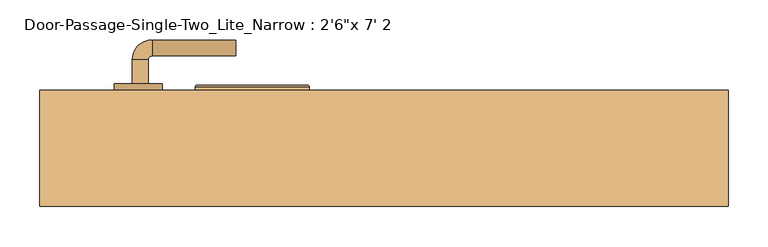
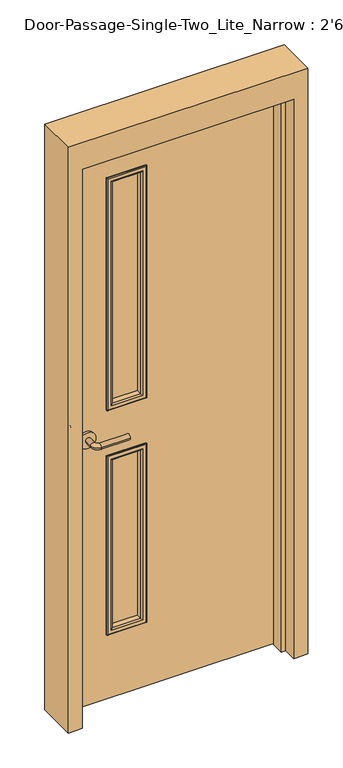
"""IFC4 building model written with IfcOpenShell, lengths in millimetres: door geometry."""

from ifc_helpers import new_model, si_unit, point, frame, frame_2d, origin, place, context, project, spatial, polyline, circle_curve, ellipse_curve, trimmed, segment, composite_curve, outline, extrude, faceted_brep, source, transform, mapped, element, save
from ifc_brep_helpers import plane_surface, cylinder_surface, revolved_surface, advanced_brep


def door_10c07981(model_context):
    return source(origin(), model_context, "Body", "SolidModel", [
        advanced_brep(
        [(-315.990625, -14.35, 1016.0), (-295.990625, -14.35, 1016.0), (-295.990625, -44.35, 1016.0), (-315.990625, -44.35, 1016.0), (-290.990625, -49.35, 1016.0), (-290.990625, -69.35, 1016.0), (-185.990625, -69.35, 1016.0), (-185.990625, -49.35, 1016.0)],
        [
            (0, 1, circle_curve(frame((-305.990625, -14.35, 1016.0), z_axis=(0.0, 1.0, 0.0), x_axis=(1.0, 0.0, 0.0)), 10.0)),
            (1, 0, circle_curve(frame((-305.990625, -14.35, 1016.0), z_axis=(0.0, 1.0, 0.0), x_axis=(1.0, 0.0, 0.0)), 10.0)),
            (1, 2),
            (2, 3, circle_curve(frame((-305.990625, -44.35, 1016.0), z_axis=(0.0, 1.0, 0.0), x_axis=(1.0, 0.0, 0.0)), 10.0)),
            (3, 0),
            (3, 2, circle_curve(frame((-305.990625, -44.35, 1016.0), z_axis=(0.0, 1.0, 0.0), x_axis=(1.0, 0.0, 0.0)), 10.0)),
            (4, 5, circle_curve(frame((-290.990625, -59.35, 1016.0), z_axis=(-1.0, 0.0, 0.0), x_axis=(0.0, 1.0, 0.0)), 10.0)),
            (5, 3, circle_curve(frame((-290.990625, -44.35, 1016.0), z_axis=(0.0, 0.0, -1.0), x_axis=(-1.0, 0.0, 0.0)), 25.0)),
            (2, 4, circle_curve(frame((-290.990625, -44.35, 1016.0), z_axis=(0.0, 0.0, 1.0), x_axis=(-1.0, 0.0, 0.0)), 5.0)),
            (5, 4, circle_curve(frame((-290.990625, -59.35, 1016.0), z_axis=(-1.0, 0.0, 0.0), x_axis=(0.0, 1.0, 0.0)), 10.0)),
            (6, 7, circle_curve(frame((-185.990625, -59.35, 1016.0), z_axis=(1.0, 0.0, 0.0), x_axis=(0.0, 1.0, 0.0)), 10.0)),
            (7, 6, circle_curve(frame((-185.990625, -59.35, 1016.0), z_axis=(1.0, 0.0, 0.0), x_axis=(0.0, 1.0, 0.0)), 10.0)),
            (4, 7),
            (6, 5),
        ],
        [
            plane_surface(frame((-305.990625, -14.35, 1016.0), z_axis=(0.0, 1.0, 0.0), x_axis=(0.0, 0.0, 1.0))),
            cylinder_surface(frame((-305.990625, -14.35, 1016.0), z_axis=(0.0, 1.0, 0.0), x_axis=(1.0, 0.0, 0.0)), 10.0),
            revolved_surface(trimmed(ellipse_curve(frame((-305.990625, -44.35, 1016.0), z_axis=(0.0, -1.0, 0.0), x_axis=(1.0, 0.0, 0.0)), 10.0, 10.0), [point((-315.990625, -44.35, 1016.0))], [point((-295.990625, -44.35, 1016.0))], True, "CARTESIAN"), (-290.990625, -44.35, 1016.0), (0.0, 0.0, -1.0)),
            revolved_surface(trimmed(ellipse_curve(frame((-305.990625, -44.35, 1016.0), z_axis=(0.0, -1.0, 0.0), x_axis=(1.0, 0.0, 0.0)), 10.0, 10.0), [point((-295.990625, -44.35, 1016.0))], [point((-315.990625, -44.35, 1016.0))], True, "CARTESIAN"), (-290.990625, -44.35, 1016.0), (0.0, 0.0, -1.0)),
            plane_surface(frame((-185.990625, -59.35, 1016.0), z_axis=(1.0, 0.0, 0.0), x_axis=(0.0, 0.0, 1.0))),
            cylinder_surface(frame((-290.990625, -59.35, 1016.0), z_axis=(-1.0, 0.0, 0.0), x_axis=(0.0, 1.0, 0.0)), 10.0),
        ],
        [
            (0, [[1, 2]]),
            (1, [[3, 4, 5, -2]]),
            (1, [[-5, 6, -3, -1]]),
            (2, [[7, 8, -4, 9]]),
            (3, [[10, -9, -6, -8]]),
            (4, [[11, 12]]),
            (5, [[13, -11, 14, -7]]),
            (5, [[-14, -12, -13, -10]]),
        ],
    ),
        extrude(outline(composite_curve([segment(trimmed(circle_curve(frame_2d((1016.0, -308.490625)), 30.0), [point((1016.0, -338.490625))], [point((1016.0, -278.490625))], False, "CARTESIAN"), True, "CONTINUOUS"), segment(trimmed(circle_curve(frame_2d((1016.0, -308.490625)), 30.0), [point((1016.0, -278.490625))], [point((1016.0, -338.490625))], False, "CARTESIAN"), True, "CONTINUOUS")], self_intersect=False)), frame((0.0, -14.35, 0.0), z_axis=(0.0, 1.0, 0.0), x_axis=(0.0, 0.0, 1.0)), (0.0, 0.0, 1.0), 8.0),
        advanced_brep(
        [(-315.990625, 46.1, 1016.0), (-295.990625, 46.1, 1016.0), (-315.990625, 76.1, 1016.0), (-295.990625, 76.1, 1016.0), (-290.990625, 81.1, 1016.0), (-290.990625, 101.1, 1016.0), (-185.990625, 101.1, 1016.0), (-185.990625, 81.1, 1016.0)],
        [
            (0, 1, circle_curve(frame((-305.990625, 46.1, 1016.0), z_axis=(0.0, -1.0, 0.0), x_axis=(1.0, 0.0, 0.0)), 10.0)),
            (1, 0, circle_curve(frame((-305.990625, 46.1, 1016.0), z_axis=(0.0, -1.0, 0.0), x_axis=(1.0, 0.0, 0.0)), 10.0)),
            (0, 2),
            (2, 3, circle_curve(frame((-305.990625, 76.1, 1016.0), z_axis=(0.0, -1.0, 0.0), x_axis=(1.0, 0.0, 0.0)), 10.0)),
            (3, 1),
            (3, 2, circle_curve(frame((-305.990625, 76.1, 1016.0), z_axis=(0.0, -1.0, 0.0), x_axis=(1.0, 0.0, 0.0)), 10.0)),
            (4, 3, circle_curve(frame((-290.990625, 76.1, 1016.0), z_axis=(0.0, 0.0, 1.0), x_axis=(-1.0, 0.0, 0.0)), 5.0)),
            (2, 5, circle_curve(frame((-290.990625, 76.1, 1016.0), z_axis=(0.0, 0.0, -1.0), x_axis=(-1.0, 0.0, 0.0)), 25.0)),
            (5, 4, circle_curve(frame((-290.990625, 91.1, 1016.0), z_axis=(-1.0, 0.0, 0.0), x_axis=(0.0, -1.0, 0.0)), 10.0)),
            (4, 5, circle_curve(frame((-290.990625, 91.1, 1016.0), z_axis=(-1.0, 0.0, 0.0), x_axis=(0.0, -1.0, 0.0)), 10.0)),
            (6, 7, circle_curve(frame((-185.990625, 91.1, 1016.0), z_axis=(1.0, 0.0, 0.0), x_axis=(0.0, -1.0, 0.0)), 10.0)),
            (7, 6, circle_curve(frame((-185.990625, 91.1, 1016.0), z_axis=(1.0, 0.0, 0.0), x_axis=(0.0, -1.0, 0.0)), 10.0)),
            (5, 6),
            (7, 4),
        ],
        [
            plane_surface(frame((-305.990625, 46.1, 1016.0), z_axis=(0.0, -1.0, 0.0), x_axis=(0.0, 0.0, 1.0))),
            cylinder_surface(frame((-305.990625, 46.1, 1016.0), z_axis=(0.0, -1.0, 0.0), x_axis=(1.0, 0.0, 0.0)), 10.0),
            revolved_surface(trimmed(ellipse_curve(frame((-305.990625, 76.1, 1016.0), z_axis=(0.0, -1.0, 0.0), x_axis=(1.0, 0.0, 0.0)), 10.0, 10.0), [point((-315.990625, 76.1, 1016.0))], [point((-295.990625, 76.1, 1016.0))], True, "CARTESIAN"), (-290.990625, 76.1, 1016.0), (0.0, 0.0, -1.0)),
            revolved_surface(trimmed(ellipse_curve(frame((-305.990625, 76.1, 1016.0), z_axis=(0.0, -1.0, 0.0), x_axis=(1.0, 0.0, 0.0)), 10.0, 10.0), [point((-295.990625, 76.1, 1016.0))], [point((-315.990625, 76.1, 1016.0))], True, "CARTESIAN"), (-290.990625, 76.1, 1016.0), (0.0, 0.0, -1.0)),
            plane_surface(frame((-185.990625, 91.1, 1016.0), z_axis=(1.0, 0.0, 0.0), x_axis=(0.0, 0.0, 1.0))),
            cylinder_surface(frame((-290.990625, 91.1, 1016.0), z_axis=(-1.0, 0.0, 0.0), x_axis=(0.0, -1.0, 0.0)), 10.0),
        ],
        [
            (0, [[1, 2]]),
            (1, [[-1, 3, 4, 5]]),
            (1, [[-2, -5, 6, -3]]),
            (2, [[7, -4, 8, 9]]),
            (3, [[-8, -6, -7, 10]]),
            (4, [[11, 12]]),
            (5, [[-9, 13, -12, 14]]),
            (5, [[-10, -14, -11, -13]]),
        ],
    ),
        extrude(outline(composite_curve([segment(trimmed(circle_curve(frame_2d((1016.0, -308.490625)), 30.0), [point((1016.0, -338.490625))], [point((1016.0, -278.490625))], False, "CARTESIAN"), True, "CONTINUOUS"), segment(trimmed(circle_curve(frame_2d((1016.0, -308.490625)), 30.0), [point((1016.0, -278.490625))], [point((1016.0, -338.490625))], False, "CARTESIAN"), True, "CONTINUOUS")], self_intersect=False)), frame((0.0, 38.1, 0.0), z_axis=(0.0, 1.0, 0.0), x_axis=(0.0, 0.0, 1.0)), (0.0, 0.0, 1.0), 8.0),
        extrude(outline(polyline([(2133.6, -381.0), (0.0, -381.0), (0.0, 381.0), (2133.6, 381.0), (2133.6, -381.0)]), holes=[polyline([(1981.2, -228.6), (1981.2, -101.6), (1111.25, -101.6), (1111.25, -228.6), (1981.2, -228.6)]), polyline([(920.75, -228.6), (920.75, -101.6), (254.0, -101.6), (254.0, -228.6), (920.75, -228.6)])]), frame((0.0, -6.35, 0.0), z_axis=(0.0, 1.0, 0.0), x_axis=(0.0, 0.0, 1.0)), (0.0, 0.0, 1.0), 44.45),
        faceted_brep([(381.0, -11.1125, 0.0), (381.0, 38.1, 0.0), (431.8, 38.1, 0.0), (431.8, -107.95, 0.0), (381.0, -107.95, 0.0), (381.0, -58.7375, 0.0), (365.125, -58.7375, 0.0), (365.125, -11.1125, 0.0), (381.0, -11.1125, 2133.6), (381.0, 38.1, 2133.6), (-381.0, 38.1, 2133.6), (-381.0, 38.1, 0.0), (-431.8, 38.1, 0.0), (-431.8, 38.1, 2235.2), (431.8, 38.1, 2235.2), (431.8, -107.95, 2235.2), (-431.8, -107.95, 2235.2), (-431.8, -107.95, 0.0), (-381.0, -107.95, 0.0), (-381.0, -107.95, 2133.6), (381.0, -107.95, 2133.6), (381.0, -58.7375, 2133.6), (-381.0, -58.7375, 2133.6), (-381.0, -58.7375, 0.0), (-365.125, -58.7375, 0.0), (-365.125, -58.7375, 2117.725), (365.125, -58.7375, 2117.725), (365.125, -11.1125, 2117.725), (-365.125, -11.1125, 2117.725), (-365.125, -11.1125, 0.0), (-381.0, -11.1125, 0.0), (-381.0, -11.1125, 2133.6)], [[[0, 1, 2, 3, 4, 5, 6, 7]], [[1, 0, 8, 9]], [[2, 1, 9, 10, 11, 12, 13, 14]], [[3, 2, 14, 15]], [[4, 3, 15, 16, 17, 18, 19, 20]], [[5, 4, 20, 21]], [[6, 5, 21, 22, 23, 24, 25, 26]], [[7, 6, 26, 27]], [[0, 7, 27, 28, 29, 30, 31, 8]], [[9, 8, 31, 10]], [[20, 19, 22, 21]], [[26, 25, 28, 27]], [[12, 11, 30, 29, 24, 23, 18, 17]], [[11, 10, 31, 30]], [[13, 12, 17, 16]], [[19, 18, 23, 22]], [[25, 24, 29, 28]], [[15, 14, 13, 16]]]),
        extrude(outline(polyline([(-101.6, 12.7), (-228.6, 12.7), (-228.6, 19.05), (-101.6, 19.05), (-101.6, 12.7)])), frame((0.0, 0.0, 1111.25), z_axis=(0.0, 0.0, 1.0), x_axis=(1.0, 0.0, 0.0)), (0.0, 0.0, 1.0), 869.95),
        extrude(outline(polyline([(-101.6, 12.7), (-228.6, 12.7), (-228.6, 19.05), (-101.6, 19.05), (-101.6, 12.7)])), frame((0.0, 0.0, 254.0), z_axis=(0.0, 0.0, 1.0), x_axis=(1.0, 0.0, 0.0)), (0.0, 0.0, 1.0), 666.75),
        advanced_brep(
        [(-228.6, 19.05, 1981.2), (-228.6, 38.1, 1981.2), (-228.6, 38.1, 1111.25), (-228.6, 19.05, 1111.25), (-216.6, 39.1, 1969.2), (-216.6, 19.05, 1969.2), (-216.6, 19.05, 1123.25), (-216.6, 39.1, 1123.25), (-221.6, 44.1, 1974.2), (-221.6, 44.1, 1118.25), (-236.6, 42.1, 1989.2), (-234.6, 44.1, 1987.2), (-234.6, 44.1, 1105.25), (-236.6, 42.1, 1103.25), (-236.6, 38.1, 1989.2), (-236.6, 38.1, 1103.25), (-101.6, 38.1, 1111.25), (-101.6, 19.05, 1111.25), (-113.6, 19.05, 1123.25), (-113.6, 39.1, 1123.25), (-108.6, 44.1, 1118.25), (-95.6, 44.1, 1105.25), (-93.6, 42.1, 1103.25), (-93.6, 38.1, 1103.25), (-101.6, 38.1, 1981.2), (-101.6, 19.05, 1981.2), (-113.6, 19.05, 1969.2), (-113.6, 39.1, 1969.2), (-108.6, 44.1, 1974.2), (-95.6, 44.1, 1987.2), (-93.6, 42.1, 1989.2), (-93.6, 38.1, 1989.2)],
        [
            (0, 1),
            (1, 2),
            (2, 3),
            (3, 0),
            (4, 5),
            (5, 6),
            (6, 7),
            (7, 4),
            (8, 4, ellipse_curve(frame((-221.6, 39.1, 1974.2), z_axis=(-0.7071067811865475, 0.0, -0.7071067811865475), x_axis=(-0.7071067811865474, 0.0, 0.7071067811865476)), 7.0710678, 5.0)),
            (7, 9, ellipse_curve(frame((-221.6, 39.1, 1118.25), z_axis=(-0.7071067811865475, 0.0, 0.7071067811865475), x_axis=(0.7071067811865474, 0.0, 0.7071067811865476)), 7.0710678, 5.0)),
            (9, 8),
            (10, 11, ellipse_curve(frame((-234.6, 42.1, 1987.2), z_axis=(-0.7071067811865475, 0.0, -0.7071067811865475), x_axis=(-0.7071067811865474, 0.0, 0.7071067811865476)), 2.8284271, 2.0)),
            (11, 12),
            (12, 13, ellipse_curve(frame((-234.6, 42.1, 1105.25), z_axis=(-0.7071067811865475, 0.0, 0.7071067811865475), x_axis=(0.7071067811865474, 0.0, 0.7071067811865476)), 2.8284271, 2.0)),
            (13, 10),
            (14, 10),
            (13, 15),
            (15, 14),
            (2, 16),
            (16, 17),
            (17, 3),
            (6, 18),
            (18, 19),
            (19, 7),
            (19, 20, ellipse_curve(frame((-108.6, 39.1, 1118.25), z_axis=(-0.7071067811865475, 0.0, -0.7071067811865475), x_axis=(-0.7071067811865476, 0.0, 0.7071067811865474)), 7.0710678, 5.0)),
            (20, 9),
            (12, 21),
            (21, 22, ellipse_curve(frame((-95.6, 42.1, 1105.25), z_axis=(-0.7071067811865475, 0.0, -0.7071067811865475), x_axis=(-0.7071067811865476, 0.0, 0.7071067811865474)), 2.8284271, 2.0)),
            (22, 13),
            (22, 23),
            (23, 15),
            (16, 24),
            (24, 25),
            (25, 17),
            (18, 26),
            (26, 27),
            (27, 19),
            (27, 28, ellipse_curve(frame((-108.6, 39.1, 1974.2), z_axis=(0.7071067811865475, 0.0, -0.7071067811865475), x_axis=(-0.7071067811865474, 0.0, -0.7071067811865476)), 7.0710678, 5.0)),
            (28, 20),
            (21, 29),
            (29, 30, ellipse_curve(frame((-95.6, 42.1, 1987.2), z_axis=(0.7071067811865475, 0.0, -0.7071067811865475), x_axis=(-0.7071067811865474, 0.0, -0.7071067811865476)), 2.8284271, 2.0)),
            (30, 22),
            (30, 31),
            (31, 23),
            (31, 14),
            (1, 24),
            (0, 25),
            (5, 26),
            (4, 27),
            (8, 28),
            (11, 29),
            (10, 30),
        ],
        [
            plane_surface(frame((-228.6, 38.1, 1981.2), z_axis=(-1.0, 0.0, 0.0), x_axis=(0.0, 0.0, -1.0))),
            plane_surface(frame((-216.6, 19.05, 1969.2), z_axis=(1.0, 0.0, 0.0), x_axis=(0.0, 0.0, -1.0))),
            cylinder_surface(frame((-221.6, 39.1, 1981.2), z_axis=(0.0, 0.0, 1.0), x_axis=(-1.0, 0.0, 0.0)), 5.0),
            cylinder_surface(frame((-234.6, 42.1, 1981.2), z_axis=(0.0, 0.0, 1.0), x_axis=(-1.0, 0.0, 0.0)), 2.0),
            plane_surface(frame((-236.6, 42.1, 1989.2), z_axis=(-1.0, 0.0, 0.0), x_axis=(0.0, 0.0, -1.0))),
            plane_surface(frame((-228.6, 38.1, 1111.25), z_axis=(0.0, 0.0, -1.0), x_axis=(1.0, 0.0, 0.0))),
            plane_surface(frame((-216.6, 19.05, 1123.25), z_axis=(0.0, 0.0, 1.0), x_axis=(1.0, 0.0, 0.0))),
            cylinder_surface(frame((-228.6, 39.1, 1118.25), z_axis=(-1.0, 0.0, 0.0), x_axis=(0.0, 0.0, -1.0)), 5.0),
            cylinder_surface(frame((-228.6, 42.1, 1105.25), z_axis=(-1.0, 0.0, 0.0), x_axis=(0.0, 0.0, -1.0)), 2.0),
            plane_surface(frame((-236.6, 42.1, 1103.25), z_axis=(0.0, 0.0, -1.0), x_axis=(1.0, 0.0, 0.0))),
            plane_surface(frame((-101.6, 38.1, 1111.25), z_axis=(1.0, 0.0, 0.0), x_axis=(0.0, 0.0, 1.0))),
            plane_surface(frame((-113.6, 19.05, 1123.25), z_axis=(-1.0, 0.0, 0.0), x_axis=(0.0, 0.0, 1.0))),
            cylinder_surface(frame((-108.6, 39.1, 1111.25), z_axis=(0.0, 0.0, -1.0), x_axis=(1.0, 0.0, 0.0)), 5.0),
            cylinder_surface(frame((-95.6, 42.1, 1111.25), z_axis=(0.0, 0.0, -1.0), x_axis=(1.0, 0.0, 0.0)), 2.0),
            plane_surface(frame((-93.6, 42.1, 1103.25), z_axis=(1.0, 0.0, 0.0), x_axis=(0.0, 0.0, 1.0))),
            plane_surface(frame((-93.6, 38.1, 1989.2), z_axis=(0.0, -1.0, 0.0), x_axis=(-1.0, 0.0, 0.0))),
            plane_surface(frame((-101.6, 38.1, 1981.2), z_axis=(0.0, 0.0, 1.0), x_axis=(-1.0, 0.0, 0.0))),
            plane_surface(frame((-101.6, 19.05, 1981.2), z_axis=(0.0, -1.0, 0.0), x_axis=(-1.0, 0.0, 0.0))),
            plane_surface(frame((-113.6, 19.05, 1969.2), z_axis=(0.0, 0.0, -1.0), x_axis=(-1.0, 0.0, 0.0))),
            cylinder_surface(frame((-101.6, 39.1, 1974.2), z_axis=(1.0, 0.0, 0.0), x_axis=(0.0, 0.0, 1.0)), 5.0),
            plane_surface(frame((-108.6, 44.1, 1974.2), z_axis=(0.0, 1.0, 0.0), x_axis=(-1.0, 0.0, 0.0))),
            cylinder_surface(frame((-101.6, 42.1, 1987.2), z_axis=(1.0, 0.0, 0.0), x_axis=(0.0, 0.0, 1.0)), 2.0),
            plane_surface(frame((-93.6, 42.1, 1989.2), z_axis=(0.0, 0.0, 1.0), x_axis=(-1.0, 0.0, 0.0))),
        ],
        [
            (0, [[1, 2, 3, 4]]),
            (1, [[5, 6, 7, 8]]),
            (2, [[9, -8, 10, 11]]),
            (3, [[12, 13, 14, 15]]),
            (4, [[16, -15, 17, 18]]),
            (5, [[-3, 19, 20, 21]]),
            (6, [[-7, 22, 23, 24]]),
            (7, [[-10, -24, 25, 26]]),
            (8, [[-14, 27, 28, 29]]),
            (9, [[-17, -29, 30, 31]]),
            (10, [[-20, 32, 33, 34]]),
            (11, [[-23, 35, 36, 37]]),
            (12, [[-25, -37, 38, 39]]),
            (13, [[-28, 40, 41, 42]]),
            (14, [[-30, -42, 43, 44]]),
            (15, [[-31, -44, 45, -18], [46, -32, -19, -2]]),
            (16, [[-33, -46, -1, 47]]),
            (17, [[-21, -34, -47, -4], [48, -35, -22, -6]]),
            (18, [[-36, -48, -5, 49]]),
            (19, [[-38, -49, -9, 50]]),
            (20, [[51, -40, -27, -13], [-26, -39, -50, -11]]),
            (21, [[-41, -51, -12, 52]]),
            (22, [[-43, -52, -16, -45]]),
        ],
    ),
        advanced_brep(
        [(-228.6, 12.7, 1111.25), (-228.6, -6.35, 1111.25), (-228.6, -6.35, 1981.2), (-228.6, 12.7, 1981.2), (-216.6, -7.35, 1123.25), (-216.6, 12.7, 1123.25), (-216.6, 12.7, 1969.2), (-216.6, -7.35, 1969.2), (-221.6, -12.35, 1118.25), (-221.6, -12.35, 1974.2), (-236.6, -10.35, 1103.25), (-234.6, -12.35, 1105.25), (-234.6, -12.35, 1987.2), (-236.6, -10.35, 1989.2), (-236.6, -6.35, 1103.25), (-236.6, -6.35, 1989.2), (-101.6, -6.35, 1981.2), (-101.6, 12.7, 1981.2), (-113.6, 12.7, 1969.2), (-113.6, -7.35, 1969.2), (-108.6, -12.35, 1974.2), (-95.6, -12.35, 1987.2), (-93.6, -10.35, 1989.2), (-93.6, -6.35, 1989.2), (-101.6, -6.35, 1111.25), (-101.6, 12.7, 1111.25), (-113.6, 12.7, 1123.25), (-113.6, -7.35, 1123.25), (-108.6, -12.35, 1118.25), (-95.6, -12.35, 1105.25), (-93.6, -10.35, 1103.25), (-93.6, -6.35, 1103.25)],
        [
            (0, 1),
            (1, 2),
            (2, 3),
            (3, 0),
            (4, 5),
            (5, 6),
            (6, 7),
            (7, 4),
            (8, 4, ellipse_curve(frame((-221.6, -7.35, 1118.25), z_axis=(-0.7071067811865475, 0.0, 0.7071067811865475), x_axis=(-0.7071067811865474, 0.0, -0.7071067811865476)), 7.0710678, 5.0)),
            (7, 9, ellipse_curve(frame((-221.6, -7.35, 1974.2), z_axis=(-0.7071067811865475, 0.0, -0.7071067811865475), x_axis=(0.7071067811865474, 0.0, -0.7071067811865476)), 7.0710678, 5.0)),
            (9, 8),
            (10, 11, ellipse_curve(frame((-234.6, -10.35, 1105.25), z_axis=(-0.7071067811865475, 0.0, 0.7071067811865475), x_axis=(-0.7071067811865474, 0.0, -0.7071067811865476)), 2.8284271, 2.0)),
            (11, 12),
            (12, 13, ellipse_curve(frame((-234.6, -10.35, 1987.2), z_axis=(-0.7071067811865475, 0.0, -0.7071067811865475), x_axis=(0.7071067811865474, 0.0, -0.7071067811865476)), 2.8284271, 2.0)),
            (13, 10),
            (14, 10),
            (13, 15),
            (15, 14),
            (2, 16),
            (16, 17),
            (17, 3),
            (6, 18),
            (18, 19),
            (19, 7),
            (19, 20, ellipse_curve(frame((-108.6, -7.35, 1974.2), z_axis=(-0.7071067811865475, 0.0, 0.7071067811865475), x_axis=(-0.7071067811865476, 0.0, -0.7071067811865474)), 7.0710678, 5.0)),
            (20, 9),
            (12, 21),
            (21, 22, ellipse_curve(frame((-95.6, -10.35, 1987.2), z_axis=(-0.7071067811865475, 0.0, 0.7071067811865475), x_axis=(-0.7071067811865476, 0.0, -0.7071067811865474)), 2.8284271, 2.0)),
            (22, 13),
            (22, 23),
            (23, 15),
            (16, 24),
            (24, 25),
            (25, 17),
            (18, 26),
            (26, 27),
            (27, 19),
            (27, 28, ellipse_curve(frame((-108.6, -7.35, 1118.25), z_axis=(0.7071067811865475, 0.0, 0.7071067811865475), x_axis=(-0.7071067811865474, 0.0, 0.7071067811865476)), 7.0710678, 5.0)),
            (28, 20),
            (21, 29),
            (29, 30, ellipse_curve(frame((-95.6, -10.35, 1105.25), z_axis=(0.7071067811865475, 0.0, 0.7071067811865475), x_axis=(-0.7071067811865474, 0.0, 0.7071067811865476)), 2.8284271, 2.0)),
            (30, 22),
            (30, 31),
            (31, 23),
            (31, 14),
            (1, 24),
            (0, 25),
            (5, 26),
            (4, 27),
            (8, 28),
            (11, 29),
            (10, 30),
        ],
        [
            plane_surface(frame((-228.6, -6.35, 1111.25), z_axis=(-1.0, 0.0, 0.0), x_axis=(0.0, 0.0, 1.0))),
            plane_surface(frame((-216.6, 12.7, 1123.25), z_axis=(1.0, 0.0, 0.0), x_axis=(0.0, 0.0, 1.0))),
            cylinder_surface(frame((-221.6, -7.35, 1111.25), z_axis=(0.0, 0.0, -1.0), x_axis=(-1.0, 0.0, 0.0)), 5.0),
            cylinder_surface(frame((-234.6, -10.35, 1111.25), z_axis=(0.0, 0.0, -1.0), x_axis=(-1.0, 0.0, 0.0)), 2.0),
            plane_surface(frame((-236.6, -10.35, 1103.25), z_axis=(-1.0, 0.0, 0.0), x_axis=(0.0, 0.0, 1.0))),
            plane_surface(frame((-228.6, -6.35, 1981.2), z_axis=(0.0, 0.0, 1.0), x_axis=(1.0, 0.0, 0.0))),
            plane_surface(frame((-216.6, 12.7, 1969.2), z_axis=(0.0, 0.0, -1.0), x_axis=(1.0, 0.0, 0.0))),
            cylinder_surface(frame((-228.6, -7.35, 1974.2), z_axis=(-1.0, 0.0, 0.0), x_axis=(0.0, 0.0, 1.0)), 5.0),
            cylinder_surface(frame((-228.6, -10.35, 1987.2), z_axis=(-1.0, 0.0, 0.0), x_axis=(0.0, 0.0, 1.0)), 2.0),
            plane_surface(frame((-236.6, -10.35, 1989.2), z_axis=(0.0, 0.0, 1.0), x_axis=(1.0, 0.0, 0.0))),
            plane_surface(frame((-101.6, -6.35, 1981.2), z_axis=(1.0, 0.0, 0.0), x_axis=(0.0, 0.0, -1.0))),
            plane_surface(frame((-113.6, 12.7, 1969.2), z_axis=(-1.0, 0.0, 0.0), x_axis=(0.0, 0.0, -1.0))),
            cylinder_surface(frame((-108.6, -7.35, 1981.2), z_axis=(0.0, 0.0, 1.0), x_axis=(1.0, 0.0, 0.0)), 5.0),
            cylinder_surface(frame((-95.6, -10.35, 1981.2), z_axis=(0.0, 0.0, 1.0), x_axis=(1.0, 0.0, 0.0)), 2.0),
            plane_surface(frame((-93.6, -10.35, 1989.2), z_axis=(1.0, 0.0, 0.0), x_axis=(0.0, 0.0, -1.0))),
            plane_surface(frame((-93.6, -6.35, 1103.25), z_axis=(0.0, 1.0, 0.0), x_axis=(-1.0, 0.0, 0.0))),
            plane_surface(frame((-101.6, -6.35, 1111.25), z_axis=(0.0, 0.0, -1.0), x_axis=(-1.0, 0.0, 0.0))),
            plane_surface(frame((-101.6, 12.7, 1111.25), z_axis=(0.0, 1.0, 0.0), x_axis=(-1.0, 0.0, 0.0))),
            plane_surface(frame((-113.6, 12.7, 1123.25), z_axis=(0.0, 0.0, 1.0), x_axis=(-1.0, 0.0, 0.0))),
            cylinder_surface(frame((-101.6, -7.35, 1118.25), z_axis=(1.0, 0.0, 0.0), x_axis=(0.0, 0.0, -1.0)), 5.0),
            plane_surface(frame((-108.6, -12.35, 1118.25), z_axis=(0.0, -1.0, 0.0), x_axis=(-1.0, 0.0, 0.0))),
            cylinder_surface(frame((-101.6, -10.35, 1105.25), z_axis=(1.0, 0.0, 0.0), x_axis=(0.0, 0.0, -1.0)), 2.0),
            plane_surface(frame((-93.6, -10.35, 1103.25), z_axis=(0.0, 0.0, -1.0), x_axis=(-1.0, 0.0, 0.0))),
        ],
        [
            (0, [[1, 2, 3, 4]]),
            (1, [[5, 6, 7, 8]]),
            (2, [[9, -8, 10, 11]]),
            (3, [[12, 13, 14, 15]]),
            (4, [[16, -15, 17, 18]]),
            (5, [[-3, 19, 20, 21]]),
            (6, [[-7, 22, 23, 24]]),
            (7, [[-10, -24, 25, 26]]),
            (8, [[-14, 27, 28, 29]]),
            (9, [[-17, -29, 30, 31]]),
            (10, [[-20, 32, 33, 34]]),
            (11, [[-23, 35, 36, 37]]),
            (12, [[-25, -37, 38, 39]]),
            (13, [[-28, 40, 41, 42]]),
            (14, [[-30, -42, 43, 44]]),
            (15, [[-31, -44, 45, -18], [46, -32, -19, -2]]),
            (16, [[-33, -46, -1, 47]]),
            (17, [[-21, -34, -47, -4], [48, -35, -22, -6]]),
            (18, [[-36, -48, -5, 49]]),
            (19, [[-38, -49, -9, 50]]),
            (20, [[51, -40, -27, -13], [-26, -39, -50, -11]]),
            (21, [[-41, -51, -12, 52]]),
            (22, [[-43, -52, -16, -45]]),
        ],
    ),
        advanced_brep(
        [(-228.6, 19.05, 920.75), (-228.6, 38.1, 920.75), (-228.6, 38.1, 254.0), (-228.6, 19.05, 254.0), (-216.6, 39.1, 908.75), (-216.6, 19.05, 908.75), (-216.6, 19.05, 266.0), (-216.6, 39.1, 266.0), (-221.6, 44.1, 913.75), (-221.6, 44.1, 261.0), (-236.6, 42.1, 928.75), (-234.6, 44.1, 926.75), (-234.6, 44.1, 248.0), (-236.6, 42.1, 246.0), (-236.6, 38.1, 928.75), (-236.6, 38.1, 246.0), (-101.6, 38.1, 254.0), (-101.6, 19.05, 254.0), (-113.6, 19.05, 266.0), (-113.6, 39.1, 266.0), (-108.6, 44.1, 261.0), (-95.6, 44.1, 248.0), (-93.6, 42.1, 246.0), (-93.6, 38.1, 246.0), (-101.6, 38.1, 920.75), (-101.6, 19.05, 920.75), (-113.6, 19.05, 908.75), (-113.6, 39.1, 908.75), (-108.6, 44.1, 913.75), (-95.6, 44.1, 926.75), (-93.6, 42.1, 928.75), (-93.6, 38.1, 928.75)],
        [
            (0, 1),
            (1, 2),
            (2, 3),
            (3, 0),
            (4, 5),
            (5, 6),
            (6, 7),
            (7, 4),
            (8, 4, ellipse_curve(frame((-221.6, 39.1, 913.75), z_axis=(-0.7071067811865475, 0.0, -0.7071067811865475), x_axis=(-0.7071067811865474, 0.0, 0.7071067811865476)), 7.0710678, 5.0)),
            (7, 9, ellipse_curve(frame((-221.6, 39.1, 261.0), z_axis=(-0.7071067811865475, 0.0, 0.7071067811865475), x_axis=(0.7071067811865474, 0.0, 0.7071067811865476)), 7.0710678, 5.0)),
            (9, 8),
            (10, 11, ellipse_curve(frame((-234.6, 42.1, 926.75), z_axis=(-0.7071067811865475, 0.0, -0.7071067811865475), x_axis=(-0.7071067811865474, 0.0, 0.7071067811865476)), 2.8284271, 2.0)),
            (11, 12),
            (12, 13, ellipse_curve(frame((-234.6, 42.1, 248.0), z_axis=(-0.7071067811865475, 0.0, 0.7071067811865475), x_axis=(0.7071067811865474, 0.0, 0.7071067811865476)), 2.8284271, 2.0)),
            (13, 10),
            (14, 10),
            (13, 15),
            (15, 14),
            (2, 16),
            (16, 17),
            (17, 3),
            (6, 18),
            (18, 19),
            (19, 7),
            (19, 20, ellipse_curve(frame((-108.6, 39.1, 261.0), z_axis=(-0.7071067811865475, 0.0, -0.7071067811865475), x_axis=(-0.7071067811865476, 0.0, 0.7071067811865474)), 7.0710678, 5.0)),
            (20, 9),
            (12, 21),
            (21, 22, ellipse_curve(frame((-95.6, 42.1, 248.0), z_axis=(-0.7071067811865475, 0.0, -0.7071067811865475), x_axis=(-0.7071067811865476, 0.0, 0.7071067811865474)), 2.8284271, 2.0)),
            (22, 13),
            (22, 23),
            (23, 15),
            (16, 24),
            (24, 25),
            (25, 17),
            (18, 26),
            (26, 27),
            (27, 19),
            (27, 28, ellipse_curve(frame((-108.6, 39.1, 913.75), z_axis=(0.7071067811865475, 0.0, -0.7071067811865475), x_axis=(-0.7071067811865474, 0.0, -0.7071067811865476)), 7.0710678, 5.0)),
            (28, 20),
            (21, 29),
            (29, 30, ellipse_curve(frame((-95.6, 42.1, 926.75), z_axis=(0.7071067811865475, 0.0, -0.7071067811865475), x_axis=(-0.7071067811865474, 0.0, -0.7071067811865476)), 2.8284271, 2.0)),
            (30, 22),
            (30, 31),
            (31, 23),
            (31, 14),
            (1, 24),
            (0, 25),
            (5, 26),
            (4, 27),
            (8, 28),
            (11, 29),
            (10, 30),
        ],
        [
            plane_surface(frame((-228.6, 38.1, 920.75), z_axis=(-1.0, 0.0, 0.0), x_axis=(0.0, 0.0, -1.0))),
            plane_surface(frame((-216.6, 19.05, 908.75), z_axis=(1.0, 0.0, 0.0), x_axis=(0.0, 0.0, -1.0))),
            cylinder_surface(frame((-221.6, 39.1, 920.75), z_axis=(0.0, 0.0, 1.0), x_axis=(-1.0, 0.0, 0.0)), 5.0),
            cylinder_surface(frame((-234.6, 42.1, 920.75), z_axis=(0.0, 0.0, 1.0), x_axis=(-1.0, 0.0, 0.0)), 2.0),
            plane_surface(frame((-236.6, 42.1, 928.75), z_axis=(-1.0, 0.0, 0.0), x_axis=(0.0, 0.0, -1.0))),
            plane_surface(frame((-228.6, 38.1, 254.0), z_axis=(0.0, 0.0, -1.0), x_axis=(1.0, 0.0, 0.0))),
            plane_surface(frame((-216.6, 19.05, 266.0), z_axis=(0.0, 0.0, 1.0), x_axis=(1.0, 0.0, 0.0))),
            cylinder_surface(frame((-228.6, 39.1, 261.0), z_axis=(-1.0, 0.0, 0.0), x_axis=(0.0, 0.0, -1.0)), 5.0),
            cylinder_surface(frame((-228.6, 42.1, 248.0), z_axis=(-1.0, 0.0, 0.0), x_axis=(0.0, 0.0, -1.0)), 2.0),
            plane_surface(frame((-236.6, 42.1, 246.0), z_axis=(0.0, 0.0, -1.0), x_axis=(1.0, 0.0, 0.0))),
            plane_surface(frame((-101.6, 38.1, 254.0), z_axis=(1.0, 0.0, 0.0), x_axis=(0.0, 0.0, 1.0))),
            plane_surface(frame((-113.6, 19.05, 266.0), z_axis=(-1.0, 0.0, 0.0), x_axis=(0.0, 0.0, 1.0))),
            cylinder_surface(frame((-108.6, 39.1, 254.0), z_axis=(0.0, 0.0, -1.0), x_axis=(1.0, 0.0, 0.0)), 5.0),
            cylinder_surface(frame((-95.6, 42.1, 254.0), z_axis=(0.0, 0.0, -1.0), x_axis=(1.0, 0.0, 0.0)), 2.0),
            plane_surface(frame((-93.6, 42.1, 246.0), z_axis=(1.0, 0.0, 0.0), x_axis=(0.0, 0.0, 1.0))),
            plane_surface(frame((-93.6, 38.1, 928.75), z_axis=(0.0, -1.0, 0.0), x_axis=(-1.0, 0.0, 0.0))),
            plane_surface(frame((-101.6, 38.1, 920.75), z_axis=(0.0, 0.0, 1.0), x_axis=(-1.0, 0.0, 0.0))),
            plane_surface(frame((-101.6, 19.05, 920.75), z_axis=(0.0, -1.0, 0.0), x_axis=(-1.0, 0.0, 0.0))),
            plane_surface(frame((-113.6, 19.05, 908.75), z_axis=(0.0, 0.0, -1.0), x_axis=(-1.0, 0.0, 0.0))),
            cylinder_surface(frame((-101.6, 39.1, 913.75), z_axis=(1.0, 0.0, 0.0), x_axis=(0.0, 0.0, 1.0)), 5.0),
            plane_surface(frame((-108.6, 44.1, 913.75), z_axis=(0.0, 1.0, 0.0), x_axis=(-1.0, 0.0, 0.0))),
            cylinder_surface(frame((-101.6, 42.1, 926.75), z_axis=(1.0, 0.0, 0.0), x_axis=(0.0, 0.0, 1.0)), 2.0),
            plane_surface(frame((-93.6, 42.1, 928.75), z_axis=(0.0, 0.0, 1.0), x_axis=(-1.0, 0.0, 0.0))),
        ],
        [
            (0, [[1, 2, 3, 4]]),
            (1, [[5, 6, 7, 8]]),
            (2, [[9, -8, 10, 11]]),
            (3, [[12, 13, 14, 15]]),
            (4, [[16, -15, 17, 18]]),
            (5, [[-3, 19, 20, 21]]),
            (6, [[-7, 22, 23, 24]]),
            (7, [[-10, -24, 25, 26]]),
            (8, [[-14, 27, 28, 29]]),
            (9, [[-17, -29, 30, 31]]),
            (10, [[-20, 32, 33, 34]]),
            (11, [[-23, 35, 36, 37]]),
            (12, [[-25, -37, 38, 39]]),
            (13, [[-28, 40, 41, 42]]),
            (14, [[-30, -42, 43, 44]]),
            (15, [[-31, -44, 45, -18], [46, -32, -19, -2]]),
            (16, [[-33, -46, -1, 47]]),
            (17, [[-21, -34, -47, -4], [48, -35, -22, -6]]),
            (18, [[-36, -48, -5, 49]]),
            (19, [[-38, -49, -9, 50]]),
            (20, [[51, -40, -27, -13], [-26, -39, -50, -11]]),
            (21, [[-41, -51, -12, 52]]),
            (22, [[-43, -52, -16, -45]]),
        ],
    ),
        advanced_brep(
        [(-101.6, 12.7, 920.75), (-101.6, -6.35, 920.75), (-101.6, -6.35, 254.0), (-101.6, 12.7, 254.0), (-113.6, -7.35, 908.75), (-113.6, 12.7, 908.75), (-113.6, 12.7, 266.0), (-113.6, -7.35, 266.0), (-108.6, -12.35, 913.75), (-108.6, -12.35, 261.0), (-93.6, -10.35, 928.75), (-95.6, -12.35, 926.75), (-95.6, -12.35, 248.0), (-93.6, -10.35, 246.0), (-93.6, -6.35, 928.75), (-93.6, -6.35, 246.0), (-228.6, -6.35, 254.0), (-228.6, 12.7, 254.0), (-216.6, 12.7, 266.0), (-216.6, -7.35, 266.0), (-221.6, -12.35, 261.0), (-234.6, -12.35, 248.0), (-236.6, -10.35, 246.0), (-236.6, -6.35, 246.0), (-228.6, -6.35, 920.75), (-228.6, 12.7, 920.75), (-216.6, 12.7, 908.75), (-216.6, -7.35, 908.75), (-221.6, -12.35, 913.75), (-234.6, -12.35, 926.75), (-236.6, -10.35, 928.75), (-236.6, -6.35, 928.75)],
        [
            (0, 1),
            (1, 2),
            (2, 3),
            (3, 0),
            (4, 5),
            (5, 6),
            (6, 7),
            (7, 4),
            (8, 4, ellipse_curve(frame((-108.6, -7.35, 913.75), z_axis=(0.7071067811865475, 0.0, -0.7071067811865475), x_axis=(0.7071067811865474, 0.0, 0.7071067811865476)), 7.0710678, 5.0)),
            (7, 9, ellipse_curve(frame((-108.6, -7.35, 261.0), z_axis=(0.7071067811865475, 0.0, 0.7071067811865475), x_axis=(-0.7071067811865474, 0.0, 0.7071067811865476)), 7.0710678, 5.0)),
            (9, 8),
            (10, 11, ellipse_curve(frame((-95.6, -10.35, 926.75), z_axis=(0.7071067811865475, 0.0, -0.7071067811865475), x_axis=(0.7071067811865474, 0.0, 0.7071067811865476)), 2.8284271, 2.0)),
            (11, 12),
            (12, 13, ellipse_curve(frame((-95.6, -10.35, 248.0), z_axis=(0.7071067811865475, 0.0, 0.7071067811865475), x_axis=(-0.7071067811865474, 0.0, 0.7071067811865476)), 2.8284271, 2.0)),
            (13, 10),
            (14, 10),
            (13, 15),
            (15, 14),
            (2, 16),
            (16, 17),
            (17, 3),
            (6, 18),
            (18, 19),
            (19, 7),
            (19, 20, ellipse_curve(frame((-221.6, -7.35, 261.0), z_axis=(0.7071067811865475, 0.0, -0.7071067811865475), x_axis=(0.7071067811865476, 0.0, 0.7071067811865474)), 7.0710678, 5.0)),
            (20, 9),
            (12, 21),
            (21, 22, ellipse_curve(frame((-234.6, -10.35, 248.0), z_axis=(0.7071067811865475, 0.0, -0.7071067811865475), x_axis=(0.7071067811865476, 0.0, 0.7071067811865474)), 2.8284271, 2.0)),
            (22, 13),
            (22, 23),
            (23, 15),
            (16, 24),
            (24, 25),
            (25, 17),
            (18, 26),
            (26, 27),
            (27, 19),
            (27, 28, ellipse_curve(frame((-221.6, -7.35, 913.75), z_axis=(-0.7071067811865475, 0.0, -0.7071067811865475), x_axis=(0.7071067811865474, 0.0, -0.7071067811865476)), 7.0710678, 5.0)),
            (28, 20),
            (21, 29),
            (29, 30, ellipse_curve(frame((-234.6, -10.35, 926.75), z_axis=(-0.7071067811865475, 0.0, -0.7071067811865475), x_axis=(0.7071067811865474, 0.0, -0.7071067811865476)), 2.8284271, 2.0)),
            (30, 22),
            (30, 31),
            (31, 23),
            (31, 14),
            (1, 24),
            (0, 25),
            (5, 26),
            (4, 27),
            (8, 28),
            (11, 29),
            (10, 30),
        ],
        [
            plane_surface(frame((-101.6, -6.35, 920.75), z_axis=(1.0, 0.0, 0.0), x_axis=(0.0, 0.0, -1.0))),
            plane_surface(frame((-113.6, 12.7, 908.75), z_axis=(-1.0, 0.0, 0.0), x_axis=(0.0, 0.0, -1.0))),
            cylinder_surface(frame((-108.6, -7.35, 920.75), z_axis=(0.0, 0.0, 1.0), x_axis=(1.0, 0.0, 0.0)), 5.0),
            cylinder_surface(frame((-95.6, -10.35, 920.75), z_axis=(0.0, 0.0, 1.0), x_axis=(1.0, 0.0, 0.0)), 2.0),
            plane_surface(frame((-93.6, -10.35, 928.75), z_axis=(1.0, 0.0, 0.0), x_axis=(0.0, 0.0, -1.0))),
            plane_surface(frame((-101.6, -6.35, 254.0), z_axis=(0.0, 0.0, -1.0), x_axis=(-1.0, 0.0, 0.0))),
            plane_surface(frame((-113.6, 12.7, 266.0), z_axis=(0.0, 0.0, 1.0), x_axis=(-1.0, 0.0, 0.0))),
            cylinder_surface(frame((-101.6, -7.35, 261.0), z_axis=(1.0, 0.0, 0.0), x_axis=(0.0, 0.0, -1.0)), 5.0),
            cylinder_surface(frame((-101.6, -10.35, 248.0), z_axis=(1.0, 0.0, 0.0), x_axis=(0.0, 0.0, -1.0)), 2.0),
            plane_surface(frame((-93.6, -10.35, 246.0), z_axis=(0.0, 0.0, -1.0), x_axis=(-1.0, 0.0, 0.0))),
            plane_surface(frame((-228.6, -6.35, 254.0), z_axis=(-1.0, 0.0, 0.0), x_axis=(0.0, 0.0, 1.0))),
            plane_surface(frame((-216.6, 12.7, 266.0), z_axis=(1.0, 0.0, 0.0), x_axis=(0.0, 0.0, 1.0))),
            cylinder_surface(frame((-221.6, -7.35, 254.0), z_axis=(0.0, 0.0, -1.0), x_axis=(-1.0, 0.0, 0.0)), 5.0),
            cylinder_surface(frame((-234.6, -10.35, 254.0), z_axis=(0.0, 0.0, -1.0), x_axis=(-1.0, 0.0, 0.0)), 2.0),
            plane_surface(frame((-236.6, -10.35, 246.0), z_axis=(-1.0, 0.0, 0.0), x_axis=(0.0, 0.0, 1.0))),
            plane_surface(frame((-236.6, -6.35, 928.75), z_axis=(0.0, 1.0, 0.0), x_axis=(1.0, 0.0, 0.0))),
            plane_surface(frame((-228.6, -6.35, 920.75), z_axis=(0.0, 0.0, 1.0), x_axis=(1.0, 0.0, 0.0))),
            plane_surface(frame((-228.6, 12.7, 920.75), z_axis=(0.0, 1.0, 0.0), x_axis=(1.0, 0.0, 0.0))),
            plane_surface(frame((-216.6, 12.7, 908.75), z_axis=(0.0, 0.0, -1.0), x_axis=(1.0, 0.0, 0.0))),
            cylinder_surface(frame((-228.6, -7.35, 913.75), z_axis=(-1.0, 0.0, 0.0), x_axis=(0.0, 0.0, 1.0)), 5.0),
            plane_surface(frame((-221.6, -12.35, 913.75), z_axis=(0.0, -1.0, 0.0), x_axis=(1.0, 0.0, 0.0))),
            cylinder_surface(frame((-228.6, -10.35, 926.75), z_axis=(-1.0, 0.0, 0.0), x_axis=(0.0, 0.0, 1.0)), 2.0),
            plane_surface(frame((-236.6, -10.35, 928.75), z_axis=(0.0, 0.0, 1.0), x_axis=(1.0, 0.0, 0.0))),
        ],
        [
            (0, [[1, 2, 3, 4]]),
            (1, [[5, 6, 7, 8]]),
            (2, [[9, -8, 10, 11]]),
            (3, [[12, 13, 14, 15]]),
            (4, [[16, -15, 17, 18]]),
            (5, [[-3, 19, 20, 21]]),
            (6, [[-7, 22, 23, 24]]),
            (7, [[-10, -24, 25, 26]]),
            (8, [[-14, 27, 28, 29]]),
            (9, [[-17, -29, 30, 31]]),
            (10, [[-20, 32, 33, 34]]),
            (11, [[-23, 35, 36, 37]]),
            (12, [[-25, -37, 38, 39]]),
            (13, [[-28, 40, 41, 42]]),
            (14, [[-30, -42, 43, 44]]),
            (15, [[-31, -44, 45, -18], [46, -32, -19, -2]]),
            (16, [[-33, -46, -1, 47]]),
            (17, [[-21, -34, -47, -4], [48, -35, -22, -6]]),
            (18, [[-36, -48, -5, 49]]),
            (19, [[-38, -49, -9, 50]]),
            (20, [[51, -40, -27, -13], [-26, -39, -50, -11]]),
            (21, [[-41, -51, -12, 52]]),
            (22, [[-43, -52, -16, -45]]),
        ],
    ),
    ])


if __name__ == "__main__":
    model = new_model("IFC4")
    model_context = context("Model", 3, world=origin())
    ifc_project = project(units=[si_unit("LENGTHUNIT", "METRE", prefix="MILLI")], contexts=[model_context])
    site = spatial("IfcSite", under=ifc_project)
    building = spatial("IfcBuilding", under=site)
    placement = place(None, origin())
    door_shape = door_10c07981(model_context)
    element("IfcDoor", 1, ObjectType="Door-Passage-Single-Two_Lite_Narrow : 2'6\"x 7' 2", at=placement, inside=building, context=model_context, shape_type="MappedRepresentation", body=[
        mapped(door_shape, transform((0.0, 0.0, 0.0), x_axis=(1.0, 0.0, 0.0), y_axis=(0.0, 1.0, 0.0), z_axis=(0.0, 0.0, 1.0))),
    ])
    save(model, "model.ifc")

# Revit data of these elements
# Type "Door-Passage-Single-Two_Lite_Narrow : 2'6\"x 7' 2"
#   Type Mark = "10"
#   Assembly Code = "B2030100"
#   Analytic Construction = "Wooden"
#   Thickness = 0' - 1 3/4"
#   Thermal Resistance (R) = 2.5876 (h·ft²·°F)/BTU
#   Swing Angle [instance default] = 90.00°
#   Strike Height = 3' - 4"
#   Rough Width [instance default] = 2' - 10"
#   Rough Height [instance default] = 7' - 4"
#   MFOpeningHeight [instance default] = 0' - 4"
#   MFOpeningWidth [instance default] = 0' - 4"
#   Heat Transfer Coefficient (U) = 0.3865 BTU/(h·ft²·°F)
#   Inset Calculate [instance default] = 0' - 4"
#   Masonry Inset [instance default] = 0' - 1"
#   Height = 7' - 0"
#   Width = 2' - 6"
#   Masonry Frame Depth = 0' - 5 3/4"
#   Masonry Frame [instance default] = yes
#   Function = 1
#   Dry Wall Frame [instance default] = no
#   Panel Material = Wood - Birch
#   Glazing = Glass
#   Glass Stop Material = Metal - Paint Finish - Grey
#   Frame Material = Metal - Paint Finish - Grey
#   Door Handle Material = Aluminum
#   Visual Light Transmittance = 0
#   Solar Heat Gain Coefficient = 0
#   Wall Closure = (empty or 0)
# Element 1 (IfcDoor, "Door-Passage-Single-Two_Lite_Narrow : 2'6\"x 7' 2")
#   Materials on its faces: "Metal - Paint Finish - Grey", "Aluminum", "Wood - Birch", "Glass"
# Materials
#   "Wood - Birch": class "Wood", colour RGB 166 116 52, transparency 0, Cost = 0
#   "Glass": class "Glass", colour RGB 0 128 192, transparency 0.75, Description = "Soda Lime Glass", Cost = 0
#   "Metal - Paint Finish - Grey": class "Paint", colour RGB 104 104 104, transparency 0, Cost = 0
#   "Aluminum": class "Metal", colour RGB 247 247 247, transparency 0, Description = "Aluminum 6061", Cost = 0
